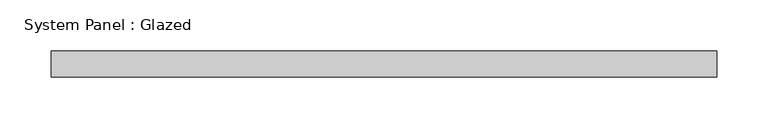
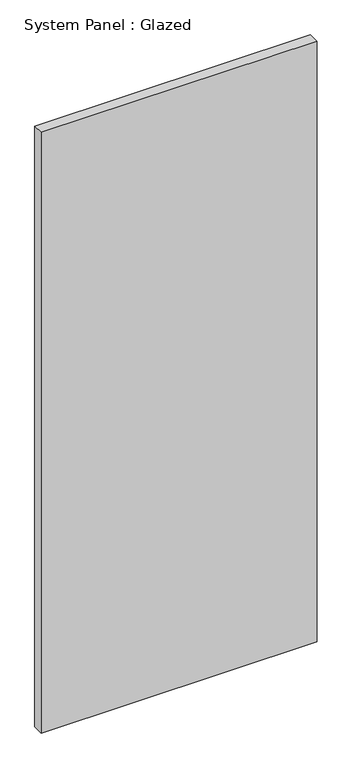
"""IFC4 building model written with IfcOpenShell, lengths in millimetres: plate geometry, System Panel : Glazed."""

from ifc_helpers import new_model, si_unit, origin, origin_with_axes, place, context, project, spatial, polyline, outline, extrude, source, transform, mapped, element, save


def system_panel_glazed_43ab5a70(model_context):
    return source(origin(), model_context, "Body", "SweptSolid", [
        extrude(outline(polyline([(323.85, 19.05), (-323.85, 19.05), (-323.85, 44.45), (323.85, 44.45), (323.85, 19.05)])), origin_with_axes(), (0.0, 0.0, 1.0), 1490.4100631),
    ])


if __name__ == "__main__":
    model = new_model("IFC4")
    model_context = context("Model", 3, world=origin())
    ifc_project = project(units=[si_unit("LENGTHUNIT", "METRE", prefix="MILLI")], contexts=[model_context])
    site = spatial("IfcSite", under=ifc_project)
    building = spatial("IfcBuilding", under=site)
    placement = place(None, origin())
    system_panel_glazed_shape = system_panel_glazed_43ab5a70(model_context)
    element("IfcPlate", 1, ObjectType="System Panel : Glazed", at=placement, inside=building, context=model_context, shape_type="MappedRepresentation", body=[
        mapped(system_panel_glazed_shape, transform((0.0, 0.0, 0.0), x_axis=(1.0, 0.0, 0.0), y_axis=(0.0, 1.0, 0.0), z_axis=(0.0, 0.0, 1.0))),
    ])
    save(model, "model.ifc")

# Revit data of these elements
# Type "System Panel : Glazed"
#   Construction Type Id = "GSP4R"
#   Analytic Construction = "1/8 in Pilkington single glazing"
#   Visual Light Transmittance = 0.9
#   Solar Heat Gain Coefficient = 0.86
#   Heat Transfer Coefficient (U) = 1.18115 BTU/(h·ft²·°F)
#   Define Thermal Properties by = 1
# Element 1 (IfcPlate, "System Panel : Glazed")
#   Materials on its faces: "Glass"
# Materials
#   "Glass": class "Glass", colour RGB 0 128 192, transparency 0.75, Description = "Soda Lime Glass", Cost = 0
